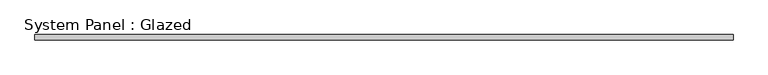
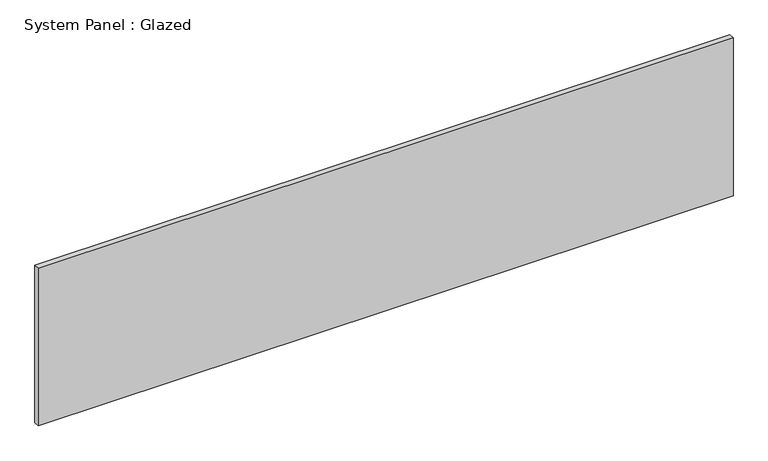
"""IFC4 building model written with IfcOpenShell, lengths in millimetres: plate geometry, System Panel : Glazed."""

from ifc_helpers import new_model, si_unit, origin, origin_with_axes, place, context, project, spatial, polyline, outline, extrude, source, transform, mapped, element, save


def system_panel_glazed_6abdcac5(model_context):
    return source(origin(), model_context, "Body", "SweptSolid", [
        extrude(outline(polyline([(1643.0382561, 19.05), (-1643.0382561, 19.05), (-1643.0382561, 44.45), (1643.0382561, 44.45), (1643.0382561, 19.05)])), origin_with_axes(), (0.0, 0.0, 1.0), 787.8042254),
    ])


if __name__ == "__main__":
    model = new_model("IFC4")
    model_context = context("Model", 3, world=origin())
    ifc_project = project(units=[si_unit("LENGTHUNIT", "METRE", prefix="MILLI")], contexts=[model_context])
    site = spatial("IfcSite", under=ifc_project)
    building = spatial("IfcBuilding", under=site)
    placement = place(None, origin())
    system_panel_glazed_shape = system_panel_glazed_6abdcac5(model_context)
    element("IfcPlate", 1, ObjectType="System Panel : Glazed", at=placement, inside=building, context=model_context, shape_type="MappedRepresentation", body=[
        mapped(system_panel_glazed_shape, transform((0.0, 0.0, 0.0), x_axis=(1.0, 0.0, 0.0), y_axis=(0.0, 1.0, 0.0), z_axis=(0.0, 0.0, 1.0))),
    ])
    save(model, "model.ifc")

# Revit data of these elements
# Type "System Panel : Glazed"
#   Construction Type Id = "GSP4R"
#   Analytic Construction = "1/8 in Pilkington single glazing"
#   Visual Light Transmittance = 0.9
#   Solar Heat Gain Coefficient = 0.86
#   Heat Transfer Coefficient (U) = 1.18115 BTU/(h·ft²·°F)
#   Define Thermal Properties by = 1
# Element 1 (IfcPlate, "System Panel : Glazed")
#   Materials on its faces: "Glass"
# Materials
#   "Glass": class "Glass", colour RGB 0 128 192, transparency 0.75, Description = "Soda Lime Glass", Cost = 0
